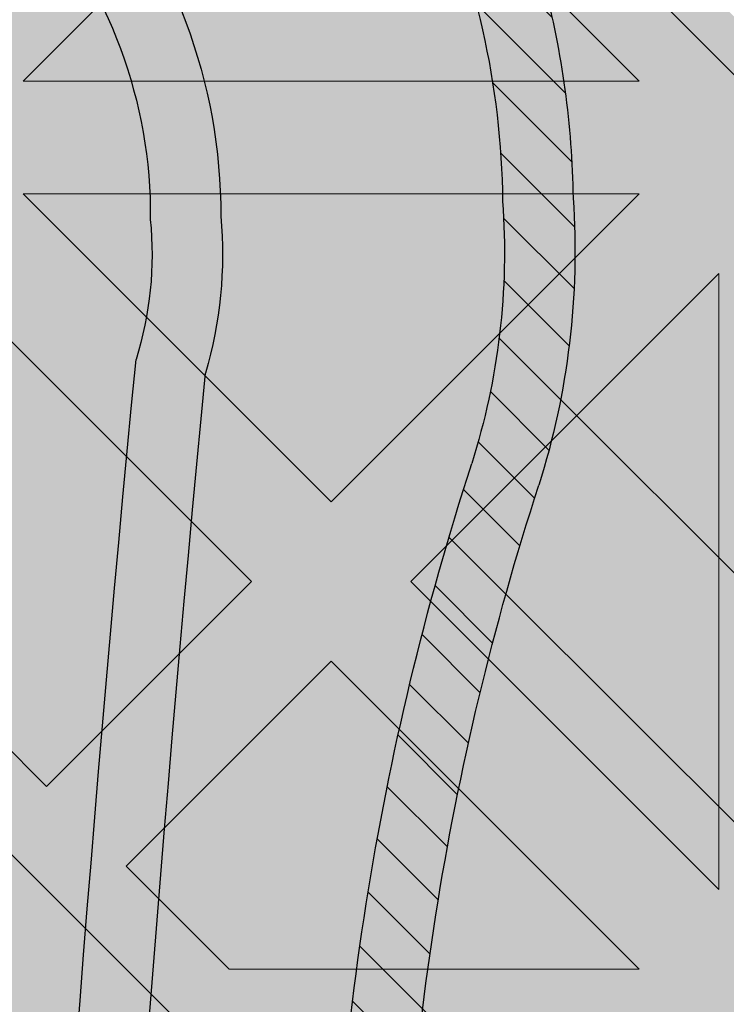
# Model space of a CAD drawing. Units: inches. Extents: x 844 to 2234, y 346 to 1084.
# Tile 78 of 93: x 1999.568 to 2001.166, y 706.514 to 708.742. Entities that reach past the tile are written whole.
import ezdxf

# ---------------------------------------------------------------- set-up
doc = ezdxf.new("R2010")
doc.units = ezdxf.units.IN
doc.header["$MEASUREMENT"] = 0
for name, color, linetype, lineweight in [('A-ANNO-DIMS', 2, 'Continuous', 18), ('furniture', 8, 'Continuous', 18), ('RA-AP-01$0$INT', 35, 'Continuous', 5)]:
    doc.layers.add(name, color=color, linetype=linetype, lineweight=lineweight)
doc.layers.add('RA-AP-01$0$FURN', color=3, linetype='Continuous')
doc.layers.add('RA-AP-01$0$WOOD', color=64, linetype='Continuous')
doc.styles.get("Standard").update_dxf_attribs({"font": 'arial.ttf'})
doc.dimstyles.get("Standard").update_dxf_attribs({"dimtxt": 6, "dimasz": 3, "dimexe": 0.18, "dimexo": 0.0625, "dimgap": 0.09, "dimtad": 0, "dimtih": 1, "dimtoh": 1, "dimdec": 1, "dimzin": 0, "dimdsep": 46, "dimlunit": 3, "dimtxsty": 'Standard', "dimblk": 'ARCHTICK', "dimcen": 0.09, "dimadec": 0, "dimazin": 0, "dimtfac": 1, "dimtdec": 1, "dimtofl": 0, "dimtmove": 0, "dimatfit": 3, "dimfxl": 1, "dimtolj": 1, "dimtzin": 0, "dimarcsym": 0})

# ---------------------------------------------------------------- blocks, each defined once
blk = doc.blocks.new('A$C18D01794')
at = {"layer": 'RA-AP-01$0$INT'}
h = blk.add_hatch(color=256, dxfattribs=at)
h.paths.add_polyline_path([(4.585917135068448, -7.856712009587804), (4.614201406330596, -7.856712009587056), (4.668846067270487, -7.802067348644738), (4.723490728212344, -7.856712009584164), (4.771774999457151, -7.856712009582887), (4.826419660396886, -7.80206734864072), (4.862780050090322, -7.838427738332541), (4.844495778842715, -7.856712009580965), (4.862780050090411, -7.856712009580482), (4.905206456960182, -7.814285602707865), (4.947632863832445, -7.856712009578238), (4.965917135079675, -7.856712009577755), (4.947632863831759, -7.838427738330656), (4.983993253523576, -7.802067348637219), (5.038637914464627, -7.856712009575829), (5.08692218571208, -7.856712009574554), (5.141566846649976, -7.802067348634224), (5.196211507589851, -7.856712009571666), (5.224495778822615, -7.856712009570916), (4.905206456953975, -7.537422687702283)])
h.paths.add_polyline_path([(4.895206456956031, -7.575706958950402), (4.895206456958921, -7.684996280828174), (4.840561796018589, -7.630351619890275)], flags=16)
h.paths.add_polyline_path([(4.915206456955638, -7.575706958949956), (4.969851117895509, -7.630351619887399), (4.915206456957609, -7.684996280827732)], flags=16)
h.paths.add_polyline_path([(4.826419660395175, -7.644493755514321), (4.881064321335613, -7.699138416452331), (4.771774999456703, -7.69913841645522)], flags=16)
h.paths.add_polyline_path([(4.983993253519558, -7.644493755510815), (5.038637914460456, -7.699138416449285), (4.929348592581548, -7.69913841645126)], flags=16)
h.paths.add_polyline_path([(4.881064321336025, -7.719138416452334), (4.826419660397532, -7.773783077393256), (4.771774999457062, -7.719138416455217)], flags=16)
h.paths.add_polyline_path([(4.929348592582019, -7.71913841645126), (5.038637914460982, -7.719138416449284), (4.983993253522945, -7.773783077389749)], flags=16)
h.paths.add_polyline_path([(4.895206456960191, -7.733280552075633), (4.895206456962115, -7.806001331460164), (4.876922185715016, -7.824285602708492), (4.840561796021581, -7.787925213016675)], flags=16)
h.paths.add_polyline_path([(4.915206456958487, -7.733280552075187), (4.969851117899527, -7.787925213013798), (4.933490728206909, -7.824285602708034), (4.9152064569598, -7.806001331461736)], flags=16)
h.paths.add_polyline_path([(4.757632863832376, -7.733280552079264), (4.812277524772842, -7.787925213017304), (4.757632863834348, -7.842569873958233)], flags=16)
h.paths.add_polyline_path([(4.737632863832376, -7.73328055207979), (4.737632863834348, -7.842569873958701), (4.682988202893906, -7.787925213020692)], flags=16)
h.paths.add_polyline_path([(5.05278005008503, -7.733280552072701), (5.052780050087917, -7.842569873951664), (4.998135389146995, -7.787925213013169)], flags=16)
h.paths.add_polyline_path([(5.072780050085024, -7.733280552072333), (5.127424711025931, -7.787925213010806), (5.072780050087916, -7.842569873951244)], flags=16)
h.paths.add_polyline_path([(4.935917135072783, -7.506712009583784), (5.255206456948811, -7.826001331459767), (5.255206456948932, -7.797717060211899), (5.200561796010279, -7.743072399273238), (5.255206456949403, -7.688427738334128), (5.25520645694961, -7.640143467086677), (5.200561796009787, -7.585498806146837), (5.236922185702417, -7.549138416454212), (5.255206456949919, -7.56742268770172), (5.255206456949998, -7.549138416454178), (5.212780050078687, -7.506712009583814), (5.25520645695036, -7.464285602712145), (5.255206456950438, -7.446001331464763), (5.236922185702424, -7.464285602712779), (5.200561796009796, -7.427925213020149), (5.255206456950753, -7.373280552079203), (5.25520645695096, -7.324996280834394), (5.200561796010322, -7.270351619893748), (5.255206456951428, -7.215706958952649), (5.255206456951547, -7.187422687705071)])
h.paths.add_polyline_path([(5.042988202883395, -7.42792521302065), (5.097632863823085, -7.373280552080975), (5.097632863822622, -7.482569873959883)], flags=16)
h.paths.add_polyline_path([(5.028846067259663, -7.442067348644384), (5.083490728198774, -7.496712009583504), (4.974201406321001, -7.496712009583035)], flags=16)
h.paths.add_polyline_path([(5.117632863823087, -7.37328055208089), (5.172277524762331, -7.42792521302015), (5.11763286382262, -7.482569873959851)], flags=16)
h.paths.add_polyline_path([(5.08349072819877, -7.516712009582191), (5.028846067259652, -7.571356670521302), (4.974201406320998, -7.516712009582638)], flags=16)
h.paths.add_polyline_path([(5.131774999446817, -7.35913841645716), (5.186419660386065, -7.413783077396415), (5.241064321325782, -7.359138416456712)], flags=17)
h.paths.add_polyline_path([(5.131774999446228, -7.496712009583703), (5.186419660386065, -7.442067348643883), (5.222780050079488, -7.478427738337313), (5.204495778832781, -7.496712009584014)], flags=16)
h.paths.add_polyline_path([(5.097632863822613, -7.530854145205813), (5.097632863823061, -7.640143467084723), (5.042988202883383, -7.585498806145032)], flags=16)
h.paths.add_polyline_path([(5.131774999446899, -7.339138416457162), (5.241064321325809, -7.339138416456712), (5.186419660386591, -7.284493755517479)], flags=17)
h.paths.add_polyline_path([(5.131774999446226, -7.516712009581999), (5.204495778830767, -7.516712009581702), (5.22278005007868, -7.534996280829206), (5.186419660386049, -7.571356670521828)], flags=16)
h.paths.add_polyline_path([(5.11763286382262, -7.530854145205852), (5.17227752476232, -7.585498806145562), (5.117632863823064, -7.64014346708481)], flags=16)
h.paths.add_polyline_path([(5.186419660386069, -7.599640941770585), (5.241064321325754, -7.654285602710281), (5.131774999446791, -7.654285602709814)], flags=16)
h.paths.add_polyline_path([(5.131774999446872, -7.674285602709813), (5.24106432132578, -7.674285602710282), (5.186419660386554, -7.728930263649504)], flags=16)
h.paths.add_polyline_path([(5.255206456951811, -7.126001331467467), (5.255206456951895, -7.106712009588038), (4.555206456956052, -7.106712009588038), (4.555206456956136, -7.12600133146746), (4.905206456953973, -7.476001331465289)])
h.paths.add_polyline_path([(4.983993253513404, -7.368930263651977), (4.92934859257295, -7.314285602713969), (5.03863791445186, -7.314285602711063)], flags=16)
h.paths.add_polyline_path([(4.969851117889988, -7.383072399276016), (4.915206456952556, -7.437717060215906), (4.915206456949648, -7.328427738338133)], flags=16)
h.paths.add_polyline_path([(4.929348592572535, -7.294285602713971), (4.983993253511019, -7.239640941773039), (5.038637914451496, -7.294285602711065)], flags=16)
h.paths.add_polyline_path([(5.052780050074912, -7.280143467087016), (4.998135389134438, -7.225498806148989), (5.052780050072919, -7.170854145208052)], flags=16)
h.paths.add_polyline_path([(5.07278005007491, -7.280143467086489), (5.072780050072918, -7.170854145207579), (5.127424711013374, -7.225498806145578)], flags=16)
h.paths.add_polyline_path([(4.89520645695295, -7.437717060216355), (4.840561796013067, -7.383072399278919), (4.895206456950961, -7.328427738338582)], flags=16)
h.paths.add_polyline_path([(4.915206456948365, -7.280143467090674), (4.915206456946434, -7.207422687704125), (4.933490728192729, -7.18913841645701), (4.969851117886972, -7.225498806149623)], flags=16)
h.paths.add_polyline_path([(4.881064321327021, -7.314285602715054), (4.82641966038902, -7.368930263655506), (4.771774999448108, -7.314285602717047)], flags=16)
h.paths.add_polyline_path([(4.895206456950073, -7.280143467091125), (4.840561796009022, -7.225498806152518), (4.876922185700835, -7.18913841645908), (4.895206456948749, -7.207422687706589)], flags=16)
h.paths.add_polyline_path([(4.983993253510392, -7.211356670525576), (4.947632863816944, -7.174996280833758), (4.965917135064043, -7.156712009585847), (5.038637914448995, -7.156712009584522)], flags=16)
h.paths.add_polyline_path([(4.881064321326543, -7.294285602715056), (4.771774999447578, -7.294285602717046), (4.826419660385607, -7.239640941776569)], flags=16)
h.paths.add_polyline_path([(4.905206456946447, -7.19913841645844), (4.862780050074785, -7.156712009587725), (4.947632863816685, -7.156712009586302)], flags=16)
h.paths.add_polyline_path([(5.14156684663679, -7.211356670521528), (5.086922185696452, -7.156712009583639), (5.196211507574223, -7.156712009581651)], flags=16)
h.paths.add_polyline_path([(4.8264196603837, -7.211356670529104), (4.771774999442643, -7.156712009590501), (4.8444957788276, -7.156712009588568), (4.862780050075511, -7.17499628083566)], flags=16)
h.paths.add_polyline_path([(4.812277524760289, -7.225498806153156), (4.757632863822258, -7.28014346709363), (4.757632863819352, -7.170854145214669)], flags=16)
h.paths.add_polyline_path([(4.73763286382226, -7.280143467093997), (4.682988202881349, -7.22549880615554), (4.737632863819352, -7.170854145215086)], flags=16)
h.paths.add_polyline_path([(4.723490728195188, -7.156712009591787), (4.668846067257299, -7.211356670532127), (4.614201406317417, -7.156712009594693)], flags=16)
h.paths.add_polyline_path([(4.597632863829262, -7.506712009583814), (4.555206456957951, -7.54913841645418), (4.555206456958029, -7.56742268770172), (4.573490728205535, -7.549138416454212), (4.609851117898167, -7.585498806146839), (4.555206456958338, -7.640143467086675), (4.555206456958546, -7.688427738334125), (4.60985111789767, -7.743072399273238), (4.555206456959015, -7.797717060211899), (4.555206456959138, -7.826001331459767), (4.874495778835167, -7.506712009583786), (4.5552064569564, -7.187422687705062), (4.555206456956523, -7.215706958952644), (4.609851117897629, -7.270351619893746), (4.555206456956988, -7.324996280834396), (4.555206456957198, -7.373280552079195), (4.609851117898153, -7.427925213020147), (4.573490728205528, -7.464285602712779), (4.555206456957507, -7.446001331464756), (4.555206456957585, -7.464285602712143)])
h.paths.add_polyline_path([(4.712780050085332, -7.482569873959882), (4.712780050084863, -7.373280552080972), (4.767424711024555, -7.42792521302065)], flags=16)
h.paths.add_polyline_path([(4.726922185709173, -7.496712009583504), (4.781566846648288, -7.442067348644384), (4.836211507586949, -7.496712009583033)], flags=16)
h.paths.add_polyline_path([(4.692780050085327, -7.482569873959851), (4.638135389145619, -7.427925213020149), (4.692780050084865, -7.373280552080892)], flags=16)
h.paths.add_polyline_path([(4.726922185709182, -7.516712009582191), (4.836211507586949, -7.51671200958264), (4.7815668466483, -7.571356670521304)], flags=16)
h.paths.add_polyline_path([(4.678637914461726, -7.496712009583706), (4.605917135075169, -7.496712009584014), (4.587632863828464, -7.478427738337311), (4.623993253521887, -7.442067348643881)], flags=16)
h.paths.add_polyline_path([(4.712780050085336, -7.530854145205816), (4.767424711024568, -7.585498806145034), (4.71278005008489, -7.640143467084724)], flags=16)
h.paths.add_polyline_path([(4.678637914461726, -7.516712009582001), (4.623993253521899, -7.571356670521829), (4.587632863829271, -7.534996280829206), (4.605917135077185, -7.5167120095817)], flags=16)
h.paths.add_polyline_path([(4.692780050085336, -7.530854145205848), (4.692780050084889, -7.64014346708481), (4.638135389145632, -7.585498806145562)], flags=16)
h.paths.add_polyline_path([(4.623993253521885, -7.413783077396415), (4.678637914461131, -7.359138416457161), (4.56934859258217, -7.359138416456712)], flags=17)
h.paths.add_polyline_path([(4.623993253521901, -7.599640941770568), (4.678637914461158, -7.654285602709814), (4.569348592582195, -7.654285602710281)], flags=16)
h.paths.add_polyline_path([(4.678637914461051, -7.339138416457162), (4.623993253521361, -7.284493755517479), (4.569348592582143, -7.339138416456712)], flags=17)
h.paths.add_polyline_path([(4.678637914461076, -7.674285602709813), (4.623993253521399, -7.728930263649504), (4.569348592582167, -7.674285602710281)], flags=16)
h = blk.add_hatch(color=256, dxfattribs=at)
h.paths.add_polyline_path([(5.028846067259997, -7.571356670520955), (4.974201406321342, -7.516712009582294), (5.083490728199115, -7.516712009581846)])
h.paths.add_polyline_path([(4.974201406321344, -7.496712009582688), (5.028846067260004, -7.442067348644037), (5.083490728199117, -7.496712009583157)])
h.paths.add_polyline_path([(5.042988202883738, -7.427925213020309), (5.097632863823428, -7.373280552080627), (5.097632863822963, -7.482569873959537)])
h.paths.add_polyline_path([(5.117632863822961, -7.482569873959509), (5.117632863823428, -7.373280552080546), (5.172277524762674, -7.427925213019804)])
h.paths.add_polyline_path([(5.131774999446572, -7.496712009583358), (5.186419660386406, -7.442067348643536), (5.222780050079831, -7.478427738336961), (5.204495778833122, -7.496712009583667)])
h.paths.add_polyline_path([(5.236922185702764, -7.464285602712433), (5.200561796010139, -7.427925213019802), (5.255206456949971, -7.373280552079975), (5.255206456950271, -7.446001331464927)])
h.paths.add_polyline_path([(5.186419660386412, -7.41378307739607), (5.131774999447164, -7.359138416456815), (5.241064321326123, -7.359138416456366)])
h.paths.add_polyline_path([(5.131774999447238, -7.339138416456815), (5.186419660386934, -7.284493755517132), (5.241064321326153, -7.339138416456368)])
h.paths.add_polyline_path([(5.200561796010663, -7.270351619893402), (5.255206456949324, -7.215706958954747), (5.255206456949777, -7.324996280832518)])
h.paths.add_polyline_path([(5.21278005007903, -7.50671200958347), (5.255206456950223, -7.464285602712278), (5.255206456950696, -7.549138416454185)])
h.paths.add_polyline_path([(5.13177499944657, -7.516712009581652), (5.204495778831106, -7.516712009581354), (5.222780050079024, -7.534996280828858), (5.186419660386397, -7.571356670521485)])
h.paths.add_polyline_path([(5.117632863823405, -7.640143467084465), (5.117632863822955, -7.530854145205498), (5.172277524762665, -7.585498806145217)])
h.paths.add_polyline_path([(5.042988202883727, -7.585498806144689), (5.097632863822957, -7.530854145205474), (5.097632863823407, -7.64014346708438)])
h.paths.add_polyline_path([(5.131774999447135, -7.654285602709467), (5.186419660386394, -7.599640941770219), (5.241064321326097, -7.654285602709933)])
h.paths.add_polyline_path([(5.200561796010128, -7.585498806146492), (5.236922185702758, -7.549138416453866), (5.255206456950264, -7.567422687701371), (5.255206456949948, -7.640143467086325)])
h.paths.add_polyline_path([(5.186419660386895, -7.728930263649157), (5.131774999447213, -7.674285602709467), (5.241064321326127, -7.674285602709934)])
h.paths.add_polyline_path([(5.200561796010624, -7.743072399272893), (5.255206456949745, -7.688427738333778), (5.255206456949276, -7.797717060211553)])
for p, q in [((5.212780050078687, -7.506712009583814), (5.255206456950353, -7.549138416454534)), ((5.131774999446228, -7.516712009581999), (5.186419660386053, -7.571356670521829)), ((5.204495778831179, -7.5167120095817), (5.131774999446228, -7.516712009581999)), ((5.204495778833082, -7.516712009584017), (5.222780050078681, -7.534996280829206)), ((5.117632863822614, -7.530854145205847), (5.172277524762319, -7.585498806145562)), ((5.117632863823062, -7.64014346708481), (5.117632863822614, -7.530854145205847)), ((5.186419660386051, -7.571356670521829), (5.222780050078681, -7.534996280829206)), ((5.200561796009783, -7.585498806146839), (5.236922185702415, -7.549138416454214)), ((5.255206456949919, -7.56742268770172), (5.236922185702415, -7.549138416454212)), ((5.117632863823062, -7.64014346708481), (5.172277524762319, -7.585498806145562)), ((5.255206456949605, -7.640143467086671), (5.200561796009783, -7.585498806146837)), ((5.131774999446792, -7.654285602709814), (5.186419660386049, -7.599640941770568)), ((5.241064321325755, -7.654285602710281), (5.186419660386049, -7.599640941770568)), ((5.131774999446792, -7.654285602709814), (5.241064321325755, -7.654285602710281)), ((5.131774999446872, -7.674285602709813), (5.241064321325782, -7.674285602710281)), ((5.18641966038655, -7.728930263649502), (5.131774999446872, -7.674285602709813)), ((5.241064321325782, -7.674285602710281), (5.186419660386552, -7.728930263649504))]:
    blk.add_line(p, q, dxfattribs=at)
blk = doc.blocks.new('A$C32926AE1')
at = {"layer": 'RA-AP-01$0$WOOD'}
h = blk.add_hatch(color=256, dxfattribs=at)
h.dxf.hatch_style = 1
h.paths.add_polyline_path([(5.157430609644524, 4.573483066760929, -0.1009492694046607), (5.155401577623758, 4.593365984175333, -0.1842662638101597), (5.172249623284174, 4.638795604568598, 0.2056608120311276), (5.179560981299304, 4.661316324430096, 0.3614336704623542), (5.134352340494423, 4.706524965234944, 0.2056608120311297), (5.111831620632933, 4.699213607219793, -0.1842662638101113), (5.066402000239693, 4.682365561559342, -0.1055311479399994), (5.045656153913092, 4.68467289944697, 0.1567636581983829), (4.763886414745334, 4.684672899446966, -0.1055311479399895), (4.743140568418733, 4.68236556155934, -0.1842662638100833), (4.6977109480255, 4.69921360721979, 0.2056608120302612), (4.675190228164109, 4.706524965234949, 0.3614336704708441), (4.629981587358889, 4.66131632442871, 0.2056608120245944), (4.637292945374126, 4.638795604567974, -0.1842662638101024), (4.654140991034615, 4.59336598417475, -0.1009492694055169), (4.652111959013835, 4.573483066760181, 0.021410119221476), (4.629748025606143, 4.156712009541676, 0.0214101192214795), (4.652111959013809, 3.739940952323101, -0.1009492694059586), (4.654140991034615, 3.720058034908448, -0.1842662638100975), (4.637292945374126, 3.674628414515226, 0.2056608120245705), (4.629981587358889, 3.652107694654492, 0.3614336704708879), (4.675190228164113, 3.606899053848249, 0.2056608120302384), (4.697710948025501, 3.614210411863408, -0.1842662638100995), (4.743140568418738, 3.63105845752386, -0.1055311479402541), (4.763886414745388, 3.628751119636215, 0.1567636581983776), (5.045656153913137, 3.628751119636244, -0.1055311479397538), (5.066402000239692, 3.631058457523857, -0.1842662638101067), (5.111831620632931, 3.614210411863407, 0.2056608120310924), (5.134352340494417, 3.606899053848256, 0.3614336704624001), (5.179560981299307, 3.652107694653103, 0.2056608120311314), (5.172249623284175, 3.6746284145146, -0.1842662638101402), (5.155401577623758, 3.72005803490786, -0.1009492694051366), (5.15743060964455, 3.739940952322354, 0.0214101192215073), (5.179794543052287, 4.156712009541468, 0.0214101192215252)])
h.paths.add_polyline_path([(4.639748609479751, 4.156712009541513, 0.0213537860821624), (4.661970494867118, 3.741887061152232, -0.094075836301374), (4.664143710413708, 3.7196126951003, -0.1824818158568985), (4.644813765429836, 3.668037719127816, 0.2056608120245319), (4.639939526753007, 3.653023905887301, 0.3614336704710246), (4.676106439397173, 3.616856993242342, 0.2056608120302234), (4.691120252638095, 3.621731231919122, -0.1824818158602558), (4.742695228611606, 3.641061176902986, -0.1029891339458722), (4.766991894714349, 3.638256818950944, 0.156709409989566), (5.042550673941472, 3.638256818950105, -0.102989133958497), (5.066847340047078, 3.641061176902949, -0.1824818158594995), (5.118422316020358, 3.621731231919103, 0.2056608120311416), (5.133436129261316, 3.616856993242346, 0.3614336704621468), (5.169603041905217, 3.653023905886178, 0.2056608120310986), (5.164728803228477, 3.668037719127177, -0.1824818158565612), (5.145398858244737, 3.719612695099578, -0.0940758363009313), (5.147572073791232, 3.741887061151398, 0.0213537860822023), (5.169793959178681, 4.156712009541451, 0.0213537860822226), (5.147572073791203, 4.571536957931898, -0.0940758363005034), (5.145398858244737, 4.59381132398362, -0.1824818158565587), (5.164728803228476, 4.645386299956021, 0.2056608120311045), (5.169603041905216, 4.66040011319702, 0.3614336704621845), (5.133436129261313, 4.696567025840856, 0.2056608120310773), (5.118422316020359, 4.691692787164098, -0.182481815859508), (5.066847340047078, 4.67236284218025, -0.1029891339584606), (5.04255067394148, 4.675167200133092, 0.156709409989566), (4.766991894714357, 4.675167200132257, -0.1029891339458842), (4.742695228611611, 4.672362842180213, -0.1824818158602725), (4.691120252638095, 4.691692787164077, 0.2056608120302152), (4.676106439397174, 4.696567025840858, 0.3614336704710363), (4.639939526753005, 4.660400113195899, 0.2056608120245495), (4.644813765429837, 4.645386299955384, -0.1824818158568934), (4.664143710413708, 4.593811323982902, -0.0940758363009187), (4.661970494867149, 4.571536957931074, 0.021353786082177)], flags=16)
h.paths.add_polyline_path([(5.129794543052235, 4.432167055276933, -0.0141661062790638), (5.130152669293814, 4.156927903047693, -0.0141661062790647), (5.129794543052234, 3.881688750818433, -0.0785247771143638), (5.10979738006795, 3.755143611847103, 0.0945969212073497), (5.105408519571111, 3.717898134952927, 0.1043170707844957), (5.116074640131521, 3.670385395016088, 0.1043170707864965), (5.068561900193738, 3.681051515576561, 0.09459692119553), (5.031316423304057, 3.676662655080835, -0.1580239521427272), (4.778226145355827, 3.676662655080367, 0.0945969211986668), (4.740980668464973, 3.681051515576592, 0.1043170707882822), (4.693467928526415, 3.670385395015844, 0.1043170707867916), (4.704134049087309, 3.717898134953662, 0.0945969211972894), (4.69974518859162, 3.755143611844042, -0.0785247771163196), (4.679748025606343, 3.881688750818406, -0.0141661062790663), (4.679389899364763, 4.156927903047693, -0.0141661062790672), (4.679748025606343, 4.432167055276998, -0.0785247771163064), (4.699745188591625, 4.55871219425134, 0.094596921197333), (4.704134049087308, 4.595957671141738, 0.1043170707867205), (4.693467928526416, 4.643470411079523, 0.1043170707882628), (4.740980668464965, 4.632804290518776, 0.0945969211988114), (4.778226145355874, 4.637193151015016, -0.158023952142669), (5.031316423304015, 4.637193151014546, 0.0945969211956361), (5.068561900193736, 4.632804290518806, 0.1043170707864979), (5.11607464013152, 4.643470411079278, 0.1043170707844617), (5.105408519571112, 4.595957671142455, 0.0945969212074597), (5.109797380067959, 4.558712194248236, -0.0785247771143467)], flags=0)
h.paths.add_polyline_path([(5.119794532311105, 4.432259799204851, -0.0142000800617244), (5.120156169157484, 4.156927903047701, -0.0142000800617277), (5.119794532311105, 3.881596006890482, -0.0784894509520253), (5.100273383573699, 3.758192358677797, 0.0940138827242913), (5.095413455884425, 3.717477693979438, 0.0606271852308753), (5.099615656341024, 3.686844378806616, 0.0606271852322524), (5.068982341167493, 3.691046579263239, 0.0940138827010453), (5.028267676478798, 3.686186651576848, -0.1580706864508061), (4.781274892180912, 3.686186651576435, 0.0940138827026903), (4.740560227491556, 3.691046579263279, 0.0606271852339895), (4.709926912317155, 3.686844378806508, 0.0606271852329405), (4.714129112773991, 3.717477693980356, 0.094013882701304), (4.709269185087677, 3.758192358669163, -0.0784894509577193), (4.689748036347473, 3.881596006890469, -0.014200080061729), (4.689386399501094, 4.156927903047709, -0.0142000800617217), (4.689748036347473, 4.432259799204808, -0.078489450957724), (4.709269185087651, 4.555663447426125, 0.0940138827014585), (4.714129112773992, 4.596378112114996, 0.0606271852329731), (4.709926912317154, 4.62701142728886, 0.0606271852340196), (4.74056022749157, 4.622809226832087, 0.0940138827024997), (4.781274892180847, 4.627669154518912, -0.1580706864508359), (5.028267676478777, 4.627669154518526, 0.0940138827010946), (5.068982341167492, 4.622809226832129, 0.060627185232254), (5.099615656341024, 4.627011427288751, 0.0606271852308727), (5.095413455884425, 4.59637811211593, 0.0940138827241088), (5.100273383573675, 4.555663447417647, -0.0784894509520978)], flags=0)
h.paths.add_polyline_path([(5.06978912287499, 4.430218106756144, -0.014241683694547), (5.070173729147532, 4.156927903047672, -0.0142416836945458), (5.06978912287499, 3.883637699339223, -0.0800609523125196), (5.052662118612511, 3.773463122773442, 0.0526421978001116), (5.04590916754064, 3.740550867606997, 0.0526421977992423), (5.012996912374707, 3.73379791653534, -0.1583028414718258), (4.796545656286308, 3.73379791653451, 0.0526421978034211), (4.763633401117837, 3.740550867607021, 0.0526421978018622), (4.756880450045755, 3.773463122774558, -0.0800609523117106), (4.739753445783639, 3.883637699339268, -0.0142416836945435), (4.739368839511098, 4.156927903047671, -0.0142416836945477), (4.739753445783639, 4.430218106756155, -0.0800609523116345), (4.75688045004574, 4.540392683320762, 0.052642197801941), (4.763633401117837, 4.573304938488346, 0.0526421978035071), (4.796545656286361, 4.580057889560873, -0.1583028414717561), (5.012996912374669, 4.580057889560039, 0.0526421977993048), (5.04590916754064, 4.57330493848837, 0.0526421978002057), (5.052662118612529, 4.540392683321868, -0.080060952312477)], flags=0)
h.paths.add_polyline_path([(5.049789715110557, 4.43038092723357, -0.0143097550741839), (5.05018085590259, 4.156927903047715, -0.0143097550741854), (5.049789715110558, 3.883474878861827, -0.0800685599149176), (5.03362098255317, 3.779581877367999, 0.0306258898956367), (5.028241146483733, 3.758218888663947, 0.0306258898977031), (5.006878157778253, 3.75283905259408, -0.1583983521624096), (4.802664410878162, 3.752839052594731, 0.0306258898946014), (4.781301422174808, 3.758218888663924, 0.0306258898967912), (4.775921586105202, 3.779581877368794, -0.080068559914251), (4.759752853548071, 3.883474878861786, -0.0143097550741854), (4.759361712756037, 4.156927903047671, -0.0143097550741854), (4.759752853548071, 4.430380927233557, -0.0800685599142479), (4.775921586105193, 4.534273928726546, 0.0306258898968306), (4.781301422174808, 4.555636917431444, 0.0306258898945754), (4.802664410878143, 4.561016753500631, -0.1583983521624168), (5.006878157778244, 4.561016753501291, 0.0306258898977177), (5.028241146483733, 4.555636917431421, 0.0306258898958182), (5.03362098255321, 4.534273928727244, -0.080068559914796)], flags=0)
h.paths.add_polyline_path([(4.999766070382627, 4.428171244713864, -0.0143443147609634), (5.000198441819402, 4.156927903047689, -0.0143443147609612), (4.999766070382627, 3.885684561381556, -0.0784641635803329), (4.987356730658798, 3.799103304488872, -0.1506053783831347), (4.822185837999821, 3.79910330448882, -0.0784641635803318), (4.809776498276007, 3.885684561381509, -0.014344314760963), (4.809344126839227, 4.156927903047677, -0.0143443147609645), (4.809776498276007, 4.428171244713873, -0.0784641635803192), (4.822185837999822, 4.514752501606549, -0.1506053783831338), (4.987356730658798, 4.514752501606494, -0.078464163580285)], flags=0)
h.paths.add_polyline_path([(4.979755254238824, 4.42764379880488, -0.0143772539198268), (4.980205517789977, 4.156927903047693, -0.0143772539198275), (4.979755254238824, 3.886212007290489, -0.0689242507424422), (4.971183264704897, 3.815276770442801, -0.1296645318904179), (4.838359303953726, 3.815276770442746, -0.0689242507424186), (4.829787314419809, 3.886212007290419, -0.0143772539198292), (4.829337050868653, 4.156927903047653, -0.0143772539198325), (4.829787314419809, 4.427643798804946, -0.0689242507424211), (4.838359303953725, 4.498579035652621, -0.1296645318904187), (4.971183264704897, 4.498579035652565, -0.0689242507424401)], flags=0)
h = blk.add_hatch(color=256, dxfattribs=at)
h.dxf.hatch_style = 1
h.paths.add_polyline_path([(5.145398858244737, 4.59381132398362, -0.1824818158565616), (5.164728803228476, 4.645386299956021, 0.2056608120311045), (5.169603041905216, 4.66040011319702, 0.3614336704621845), (5.133436129261313, 4.696567025840856, 0.2056608120310773), (5.118422316020359, 4.691692787164098, -0.182481815859508), (5.066847340047078, 4.67236284218025, -0.1029891339584606), (5.04255067394148, 4.675167200133092, 0.156709409989566), (4.766991894714357, 4.675167200132257, -0.1029891339458842), (4.742695228611611, 4.672362842180213, -0.1824818158602725), (4.691120252638095, 4.691692787164077, 0.2056608120302152), (4.676106439397174, 4.696567025840858, 0.3614336704710363), (4.639939526753005, 4.660400113195899, 0.2056608120245495), (4.644813765429837, 4.645386299955384, -0.1824818158568934), (4.664143710413708, 4.593811323982902, -0.0940758363009187), (4.661970494867149, 4.571536957931074, 0.0213537860821772), (4.639748609479751, 4.156712009541507, 0.0213537860821625), (4.661970494867119, 3.741887061152226, -0.0940758363013071), (4.664143710413708, 3.719612695100309, -0.1824818158569294), (4.644813765429836, 3.668037719127816, 0.2056608120245319), (4.639939526753007, 3.653023905887301, 0.3614336704710246), (4.676106439397173, 3.616856993242342, 0.2056608120302234), (4.691120252638095, 3.621731231919122, -0.1824818158602558), (4.742695228611606, 3.641061176902986, -0.1029891339458722), (4.766991894714349, 3.638256818950944, 0.156709409989566), (5.042550673941472, 3.638256818950105, -0.102989133958497), (5.066847340047078, 3.641061176902949, -0.1824818158594995), (5.118422316020358, 3.621731231919103, 0.2056608120311416), (5.133436129261316, 3.616856993242346, 0.3614336704621468), (5.169603041905217, 3.653023905886178, 0.2056608120310986), (5.164728803228477, 3.668037719127177, -0.1824818158565612), (5.145398858244737, 3.719612695099578, -0.0940758363009313), (5.147572073791232, 3.741887061151398, 0.0213537860822023), (5.169793959178681, 4.156712009541451, 0.0213537860822226), (5.147572073791203, 4.571536957931898, -0.0940758363004996)])
h.paths.add_polyline_path([(5.109797380067958, 4.55871219424824, -0.0785247771143472), (5.129794543052234, 4.432167055276936, -0.0141661062790644), (5.130152669293814, 4.156927903047685, -0.014166106279066), (5.129794543052234, 3.881688750818401, -0.0785247771143517), (5.109797380067946, 3.755143611847092, 0.0945969212073132), (5.105408519571111, 3.717898134952929, 0.1043170707844995), (5.116074640131521, 3.670385395016088, 0.1043170707864965), (5.068561900193738, 3.681051515576561, 0.09459692119553), (5.031316423304057, 3.676662655080835, -0.1580239521427272), (4.778226145355827, 3.676662655080367, 0.0945969211986668), (4.740980668464973, 3.681051515576592, 0.1043170707882822), (4.693467928526415, 3.670385395015844, 0.1043170707867916), (4.704134049087309, 3.717898134953662, 0.0945969211972894), (4.69974518859162, 3.755143611844042, -0.0785247771163196), (4.679748025606343, 3.881688750818406, -0.0141661062790663), (4.679389899364763, 4.156927903047693, -0.0141661062790672), (4.679748025606343, 4.432167055276998, -0.0785247771163064), (4.699745188591625, 4.55871219425134, 0.094596921197333), (4.704134049087308, 4.595957671141738, 0.1043170707867205), (4.693467928526416, 4.643470411079523, 0.1043170707882628), (4.740980668464965, 4.632804290518776, 0.0945969211988114), (4.778226145355874, 4.637193151015016, -0.158023952142669), (5.031316423304015, 4.637193151014546, 0.0945969211956361), (5.068561900193736, 4.632804290518806, 0.1043170707864979), (5.11607464013152, 4.643470411079278, 0.1043170707844617), (5.105408519571112, 4.595957671142455, 0.0945969212074504)], flags=16)
h.paths.add_polyline_path([(5.100273383573655, 4.55566344741771, -0.0784894509521388), (5.119794532311105, 4.432259799204852, -0.0142000800617252), (5.120156169157484, 4.156927903047686, -0.014200080061726), (5.119794532311105, 3.881596006890502, -0.0784894509520446), (5.100273383573696, 3.758192358677786, 0.0940138827242721), (5.095413455884425, 3.717477693979436, 0.0606271852308692), (5.099615656341024, 3.686844378806616, 0.0606271852322522), (5.068982341167493, 3.691046579263239, 0.0940138827010453), (5.028267676478798, 3.686186651576848, -0.1580706864508061), (4.781274892180912, 3.686186651576435, 0.0940138827026903), (4.740560227491556, 3.691046579263279, 0.0606271852339895), (4.709926912317155, 3.686844378806508, 0.0606271852329405), (4.714129112773991, 3.717477693980356, 0.094013882701304), (4.709269185087677, 3.758192358669163, -0.0784894509577193), (4.689748036347473, 3.881596006890469, -0.014200080061729), (4.689386399501094, 4.156927903047709, -0.0142000800617217), (4.689748036347473, 4.432259799204808, -0.078489450957724), (4.709269185087651, 4.555663447426125, 0.0940138827014585), (4.714129112773992, 4.596378112114996, 0.0606271852329731), (4.709926912317154, 4.62701142728886, 0.0606271852340196), (4.74056022749157, 4.622809226832087, 0.0940138827024997), (4.781274892180847, 4.627669154518912, -0.1580706864508359), (5.028267676478777, 4.627669154518526, 0.0940138827010946), (5.068982341167492, 4.622809226832129, 0.060627185232254), (5.099615656341024, 4.627011427288751, 0.0606271852308727), (5.095413455884425, 4.59637811211593, 0.094013882723957)], flags=0)
h.paths.add_polyline_path([(5.04590916754064, 4.57330493848837, 0.0526421978002057), (5.052662118612529, 4.540392683321868, -0.0800609523124783), (5.06978912287499, 4.430218106756142, -0.0142416836945469), (5.070173729147532, 4.156927903047672, -0.0142416836945458), (5.06978912287499, 3.883637699339223, -0.0800609523125196), (5.052662118612511, 3.773463122773442, 0.0526421978001116), (5.04590916754064, 3.740550867606997, 0.0526421977992423), (5.012996912374707, 3.73379791653534, -0.1583028414718258), (4.796545656286308, 3.73379791653451, 0.0526421978034211), (4.763633401117837, 3.740550867607021, 0.0526421978018622), (4.756880450045755, 3.773463122774558, -0.0800609523117106), (4.739753445783639, 3.883637699339268, -0.0142416836945435), (4.739368839511098, 4.156927903047671, -0.0142416836945477), (4.739753445783639, 4.430218106756155, -0.0800609523116345), (4.75688045004574, 4.540392683320762, 0.052642197801941), (4.763633401117837, 4.573304938488346, 0.0526421978035071), (4.796545656286361, 4.580057889560873, -0.1583028414717561), (5.012996912374669, 4.580057889560039, 0.0526421977993048)], flags=0)
h.paths.add_polyline_path([(5.028241146483733, 4.555636917431422, 0.0306258898956949), (5.033620982553182, 4.534273928727329, -0.0800685599148649), (5.049789715110557, 4.430380927233569, -0.0143097550741839), (5.05018085590259, 4.156927903047715, -0.0143097550741854), (5.049789715110558, 3.883474878861827, -0.0800685599149176), (5.03362098255317, 3.779581877367999, 0.0306258898956367), (5.028241146483733, 3.758218888663947, 0.0306258898977031), (5.006878157778253, 3.75283905259408, -0.1583983521624096), (4.802664410878162, 3.752839052594731, 0.0306258898946014), (4.781301422174808, 3.758218888663924, 0.0306258898967912), (4.775921586105202, 3.779581877368794, -0.080068559914251), (4.759752853548071, 3.883474878861786, -0.0143097550741854), (4.759361712756037, 4.156927903047671, -0.0143097550741854), (4.759752853548071, 4.430380927233557, -0.0800685599142479), (4.775921586105193, 4.534273928726546, 0.0306258898968306), (4.781301422174808, 4.555636917431444, 0.0306258898945754), (4.802664410878143, 4.561016753500631, -0.1583983521624168), (5.006878157778244, 4.561016753501291, 0.0306258898977174)], flags=0)
h.paths.add_polyline_path([(4.987356730658798, 4.514752501606494, -0.0784641635803018), (4.999766070382627, 4.428171244713845, -0.0143443147609637), (5.000198441819402, 4.156927903047665, -0.0143443147609622), (4.999766070382628, 3.885684561381514, -0.0784641635802952), (4.987356730658797, 3.799103304488872, -0.1506053783831338), (4.822185837999821, 3.799103304488819, -0.0784641635803342), (4.809776498276007, 3.885684561381512, -0.0143443147609628), (4.809344126839227, 4.156927903047676, -0.0143443147609646), (4.809776498276007, 4.428171244713873, -0.0784641635803192), (4.822185837999822, 4.514752501606549, -0.1506053783831338)], flags=0)
h.paths.add_polyline_path([(4.971183264704897, 4.498579035652566, -0.0689242507424384), (4.979755254238824, 4.427643798804883, -0.0143772539198276), (4.980205517789977, 4.15692790304768, -0.0143772539198258), (4.979755254238823, 3.88621200729051, -0.0689242507424628), (4.971183264704897, 3.815276770442801, -0.129664531890417), (4.838359303953726, 3.815276770442746, -0.0689242507424186), (4.829787314419809, 3.886212007290419, -0.0143772539198292), (4.829337050868653, 4.156927903047653, -0.0143772539198325), (4.829787314419809, 4.427643798804946, -0.0689242507424211), (4.838359303953725, 4.498579035652621, -0.1296645318904187)], flags=0)
h = blk.add_hatch(dxfattribs=at)
h.set_pattern_fill('ANSI31', color=256, scale=0.05, style=0)
h.set_pattern_definition([(45, (0, 0), (-0.0044194173824159, 0.0044194173824159), [])])
h.paths.add_polyline_path([(5.130152669293814, 4.156927903047704, 0.0141661062790657), (5.129794543052234, 4.432167055276982, 0.0777827904001433), (5.110168979996553, 4.557559993161921, -0.0976515123401879), (5.105408519571111, 4.595957671142454, -0.1043170707844687), (5.116074640131522, 4.64347041107928), (5.099615656341024, 4.627011427288751, 0.0606271852308727), (5.095413455884425, 4.59637811211593, 0.0940138827241088), (5.100273383573675, 4.555663447417647, -0.0784894509520972), (5.119794532311105, 4.432259799204852, -0.0142000800617252), (5.120156169157484, 4.156927903047686, -0.014200080061726), (5.119794532311105, 3.881596006890502, -0.0784894509520446), (5.100273383573696, 3.758192358677786, 0.0940138827242721), (5.095413455884425, 3.717477693979436, 0.0606271852308692), (5.099615656341024, 3.686844378806616), (5.116074640131519, 3.67038539501609, -0.1043170707844594), (5.105408519571112, 3.717898134952912, -0.0976515123401594), (5.11016897999655, 3.756295812933435, 0.0777827904001654), (5.129794543052234, 3.881688750818409, 0.0141661062790665)])
h.paths.add_polyline_path([(5.030164222210597, 3.676291055149937, -0.0976515123472002), (5.068561900193739, 3.681051515576561, -0.1043170707864927), (5.116074640131521, 3.670385395016088), (5.099615656341024, 3.686844378806616, 0.0606271852322522), (5.068982341167493, 3.691046579263239, 0.0940138827010453), (5.028267676478798, 3.686186651576848, -0.1580706864508061), (4.781274892180912, 3.686186651576435, 0.0940138827026903), (4.740560227491556, 3.691046579263279, 0.0606271852339913), (4.709926912317154, 3.686844378806508), (4.693467928526416, 3.670385395015845, -0.1043170707882796), (4.740980668464973, 3.681051515576592, -0.0976515123427246), (4.779378346446416, 3.676291055150394, 0.156512506893803)])
h.paths.add_polyline_path([(4.689748036347473, 3.881596006890472, -0.014200080061729), (4.689386399501094, 4.156927903047712, -0.0142000800617195), (4.689748036347473, 4.432259799204768, -0.078489450957742), (4.709269185087648, 4.555663447426114, 0.0940138827014821), (4.714129112773992, 4.596378112114995, 0.0606271852329748), (4.709926912317154, 4.62701142728886), (4.693467928526414, 4.643470411079524, -0.1043170707867939), (4.704134049087309, 4.595957671141706, -0.09765151234893), (4.699373588660725, 4.557559993157876, 0.0777827903975372), (4.679748025606343, 4.432167055276987, 0.0141661062790675), (4.679389899364763, 4.156927903047675, 0.0141661062790641), (4.679748025606343, 3.88168875081843, 0.0777827903975637), (4.699373588660724, 3.756295812937497, -0.0976515123490278), (4.704134049087308, 3.717898134953629, -0.1043170707867196), (4.693467928526416, 3.670385395015845), (4.709926912317155, 3.686844378806508, 0.0606271852329413), (4.714129112773991, 3.717477693980357, 0.0940138827013084), (4.709269185087676, 3.758192358669166, -0.0784894509577192)])
h.paths.add_polyline_path([(4.779378346446434, 4.63756475094498, -0.0976515123427943), (4.740980668464964, 4.632804290518776, -0.1043170707882609), (4.693467928526416, 4.643470411079523), (4.709926912317154, 4.62701142728886, 0.0606271852340196), (4.74056022749157, 4.622809226832087, 0.0940138827024997), (4.781274892180847, 4.627669154518912, -0.1580706864508359), (5.028267676478777, 4.627669154518526, 0.0940138827010946), (5.068982341167492, 4.622809226832129, 0.060627185232254), (5.099615656341024, 4.627011427288751), (5.116074640131521, 4.643470411079279, -0.1043170707865022), (5.068561900193735, 4.632804290518806, -0.0976515123475899), (5.030164222210446, 4.637564750945479, 0.1565125068936924)])
h = blk.add_hatch(dxfattribs=at)
h.set_pattern_fill('ANSI32', color=256, scale=0.2, style=0)
h.set_pattern_definition([(45, (0, 0), (-0.0530330085889911, 0.0530330085889911), []), (45, (0.035355339, 0), (-0.0530330085889911, 0.0530330085889911), [])])
h.paths.add_polyline_path([(5.119794532311105, 4.432259799204823, 0.0777015974868765), (5.10065834347252, 4.554469821747928, -0.0968902511992216), (5.095413455884425, 4.596378112115931, -0.060627185230871), (5.099615656341024, 4.627011427288751, -0.060627185232254), (5.068982341167492, 4.622809226832129, -0.0968902512198245), (5.027074050790956, 4.628054114423209, 0.1564657949319105), (4.782468517866163, 4.628054114422785, -0.0968902512152247), (4.740560227491555, 4.622809226832088, -0.0606271852339878), (4.709926912317155, 4.627011427288859, -0.0606271852329413), (4.714129112773991, 4.596378112115011, -0.0968902512205338), (4.708884225182929, 4.554469821738175, 0.0777015974804443), (4.689748036347473, 4.43225979920482, 0.0142000800617215), (4.689386399501094, 4.156927903047726, 0.0142000800617273), (4.689748036347473, 3.88159600689052, 0.077701597480541), (4.708884225182985, 3.759385984357019, -0.096890251220082), (4.714129112773992, 3.717477693980371, -0.0606271852329731), (4.709926912317154, 3.686844378806507, -0.060627185233988), (4.740560227491554, 3.691046579263279, -0.0968902512152569), (4.782468517866175, 3.685801691672578, 0.1564657949319236), (5.027074050790988, 3.685801691672169, -0.0968902512197451), (5.068982341167491, 3.691046579263239, -0.0606271852322557), (5.099615656341024, 3.686844378806616, -0.0606271852308727), (5.095413455884425, 3.717477693979438, -0.0968902511991229), (5.100658343472507, 3.7593859843474, 0.0777015974868745), (5.119794532311105, 3.8815960068905, 0.014200080061726), (5.120156169157484, 4.156927903047685, 0.0142000800617238)])
h.paths.add_polyline_path([(5.070173729147531, 4.156927903047684, -0.0142416836945481), (5.06978912287499, 3.883637699339191, -0.0800609523125107), (5.052662118612505, 3.773463122773424, 0.0526421978000811), (5.04590916754064, 3.740550867606997, 0.0526421977993214), (5.012996912374658, 3.733797916535325, -0.1583028414717916), (4.796545656286304, 3.733797916534512, 0.0526421978034138), (4.763633401117837, 3.740550867607021, 0.0526421978018622), (4.756880450045755, 3.773463122774558, -0.0800609523117106), (4.739753445783639, 3.883637699339268, -0.0142416836945435), (4.739368839511098, 4.156927903047671, -0.0142416836945477), (4.739753445783639, 4.430218106756155, -0.0800609523116345), (4.75688045004574, 4.540392683320762, 0.052642197801941), (4.763633401117837, 4.573304938488346, 0.0526421978035071), (4.796545656286361, 4.580057889560873, -0.1583028414717561), (5.012996912374669, 4.580057889560039, 0.0526421977993048), (5.04590916754064, 4.57330493848837, 0.0526421978002057), (5.052662118612529, 4.540392683321868, -0.0800609523124783), (5.06978912287499, 4.430218106756142, -0.0142416836945463)], flags=16)
h.paths.add_polyline_path([(5.050180855902591, 4.156927903047686, -0.0143097550741856), (5.049789715110558, 3.883474878861795, -0.0800685599148126), (5.033620982553202, 3.7795818773681, 0.0306258898957837), (5.028241146483733, 3.758218888663947, 0.0306258898977031), (5.006878157778253, 3.75283905259408, -0.1583983521624096), (4.802664410878162, 3.752839052594731, 0.0306258898946014), (4.781301422174808, 3.758218888663924, 0.0306258898967912), (4.775921586105202, 3.779581877368794, -0.080068559914251), (4.759752853548071, 3.883474878861786, -0.0143097550741854), (4.759361712756037, 4.156927903047671, -0.0143097550741854), (4.759752853548071, 4.430380927233557, -0.0800685599142479), (4.775921586105193, 4.534273928726546, 0.0306258898968306), (4.781301422174808, 4.555636917431444, 0.0306258898945754), (4.802664410878143, 4.561016753500631, -0.1583983521624168), (5.006878157778244, 4.561016753501291, 0.0306258898977177), (5.028241146483733, 4.555636917431421, 0.0306258898958182), (5.03362098255321, 4.534273928727244, -0.0800685599147973), (5.049789715110557, 4.430380927233568, -0.0143097550741854)], flags=0)
h.paths.add_polyline_path([(5.000198441819402, 4.15692790304769, -0.0143443147609622), (4.999766070382627, 3.885684561381539, -0.0784641635803169), (4.987356730658798, 3.799103304488873, -0.1506053783831347), (4.822185837999821, 3.79910330448882, -0.0784641635803318), (4.809776498276007, 3.885684561381509, -0.014344314760963), (4.809344126839227, 4.156927903047677, -0.0143443147609645), (4.809776498276007, 4.428171244713873, -0.0784641635803192), (4.822185837999822, 4.514752501606549, -0.1506053783831338), (4.987356730658798, 4.514752501606494, -0.0784641635803018), (4.999766070382627, 4.428171244713845, -0.0143443147609624)], flags=0)
h.paths.add_polyline_path([(4.980205517789976, 4.156927903047707, -0.0143772539198295), (4.979755254238824, 3.886212007290466, -0.06892425074242), (4.971183264704897, 3.815276770442801, -0.129664531890417), (4.838359303953726, 3.815276770442746, -0.0689242507424186), (4.829787314419809, 3.886212007290419, -0.0143772539198292), (4.829337050868653, 4.156927903047653, -0.0143772539198325), (4.829787314419809, 4.427643798804946, -0.0689242507424211), (4.838359303953725, 4.498579035652621, -0.1296645318904187), (4.971183264704897, 4.498579035652565, -0.0689242507424418), (4.979755254238824, 4.427643798804878, -0.0143772539198259)], flags=0)
for centre, radius, start, end in [((5.223368649208389, 4.593998637499738), 0.0779700159629894, 138.7710509204691, 180.1376463004422), ((5.223368649208376, 4.594430424511923), 0.117970015963001, 155.4366730502991, 179.2582248126249), ((5.223368649208353, 4.593998637499641), 0.067970015963027, 138.7710509203988, 180.5333070514128), ((5.223368649208383, 4.594430424511894), 0.127970015963015, 165.2501910273334, 179.1279317463626), ((5.205154176610191, 4.588829985555065), 0.1099999999999514, 176.0653099106177, 197.5485591654358), ((5.205154176610212, 4.588829985554959), 0.0999999999999796, 175.9126711156995, 197.5283650464391), ((5.205154176610212, 4.588398198542794), 0.0599999999999777, 174.823807838761, 196.3211313301264), ((5.205154176610233, 4.588398198542771), 0.0500000000000019, 174.2979292346878, 197.3556839753019), ((0.304323780376417, 4.104079819130551), 4.875754844654793, 0.6185013483537143, 5.524589681839913), ((0.304323780376417, 4.104079819130551), 4.865754844654794, 0.6185013483537143, 5.512956158076888), ((4.719397359771062, 4.432167055276791), 0.4103971832811724, 2.64254e-11, 17.95969975512227), ((4.719397359771062, 4.432167055276791), 0.4003971832811724, 2.64254e-11, 17.95969975512227)]:
    blk.add_arc(centre, radius, start, end, dxfattribs=at)
blk = doc.blocks.new('A$C5D2F253E')
at = {"layer": 'RA-AP-01$0$FURN', "xscale": -0.7999999999883585, "yscale": 0.7999999999883585, "zscale": 0.8, "rotation": 90}
blk.add_blockref('A$C18D01794', (-5.687757199772477, 4.75791982714071), dxfattribs=at)
at = {"layer": 'RA-AP-01$0$WOOD', "rotation": 270}
blk.add_blockref('A$C32926AE1', (-4.161339601644158, 5.73852594588169), dxfattribs=at)
blk = doc.blocks.new('_ArchTick')
at = {"color": 0, "linetype": 'ByBlock', "const_width": 0.15}
blk.add_lwpolyline([(-0.5, -0.5), (0.5, 0.5)], dxfattribs=at)
blk = doc.blocks.new('*D121')
at = {"layer": 'A-ANNO-DIMS', "color": 0, "lineweight": -2, "transparency": 16777216}
for p, q in [((2030.271987351997, 734.262611118704), (2040.245275089302, 734.262611118704)), ((2040.065275089302, 734.262611118704), (2040.065275089302, 704.6043509484256)), ((2040.065275089302, 668.557359536674), (2040.065275089302, 698.2156197069523)), ((2030.271987351997, 668.557359536674), (2040.245275089302, 668.557359536674))]:
    blk.add_line(p, q, dxfattribs=at)
at = {"layer": 'Defpoints', "color": 0, "transparency": 16777216}
for p in [(2030.209487351997, 734.262611118704), (2040.065275089302, 734.262611118704), (2030.209487351997, 668.557359536674)]:
    blk.add_point(p, dxfattribs=at)
at = {"layer": 'A-ANNO-DIMS', "color": 0, "lineweight": -2, "transparency": 16777216, "xscale": 3, "yscale": 3, "zscale": 3}
for p, rotation in [((2040.065275089302, 734.262611118704), 90), ((2040.065275089302, 668.557359536674), 270)]:
    blk.add_blockref('_ArchTick', p, dxfattribs=dict(at, rotation=rotation))
at = {"layer": 'A-ANNO-DIMS', "color": 0, "transparency": 16777216, "insert": (2040.065275089302, 701.4099853276883), "char_height": 6, "attachment_point": 5}
blk.add_mtext('\\A1;LOUNGE SET 5\'-5 1/2" TYP.', dxfattribs=at)

msp = doc.modelspace()

# ---------------------------------------------------------------- block references
at = {"layer": 'furniture', "xscale": -15.94108302203742, "yscale": 15.94108302203742, "zscale": 15.94108302203742, "rotation": 270}
msp.add_blockref('A$C5D2F253E', (1990.567271852805, 701.4028671565849), dxfattribs=at)

# ---------------------------------------------------------------- dimensions: what is measured, and where the dimension line sits
at = {"layer": 'A-ANNO-DIMS'}
dim = msp.add_linear_dim(base=(2040.065275089302, 734.262611118704), p1=(2030.209487351996, 668.5573595366737), p2=(2030.209487351996, 734.2626111187037), angle=90, text='LOUNGE SET <> TYP.', dimstyle='Standard', override={"dimdec": 1, "dimlfac": 1, "dimrnd": 0, "dimzin": 1, "dimdsep": 46, "dimlunit": 4, "dimfrac": 2}, dxfattribs=at)
dim.commit()
dim.dimension.update_dxf_attribs({"geometry": '*D121', "text_midpoint": (2040.065275089302, 701.4099853276883)})

doc.saveas('drawing.dxf')
